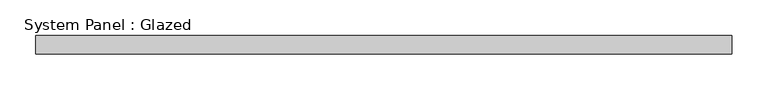
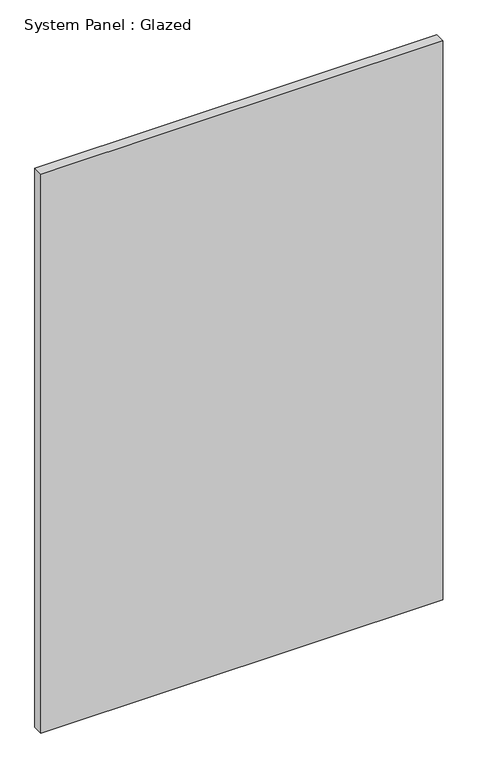
"""IFC4 building model written with IfcOpenShell, lengths in millimetres: plate geometry, System Panel : Glazed."""

from ifc_helpers import new_model, si_unit, origin, origin_with_axes, place, context, project, spatial, polyline, outline, extrude, source, transform, mapped, element, save


def system_panel_glazed_a8655be6(model_context):
    return source(origin(), model_context, "Body", "SweptSolid", [
        extrude(outline(polyline([(485.775, 19.05), (-485.775, 19.05), (-485.775, 44.45), (485.775, 44.45), (485.775, 19.05)])), origin_with_axes(), (0.0, 0.0, 1.0), 1428.75),
    ])


if __name__ == "__main__":
    model = new_model("IFC4")
    model_context = context("Model", 3, world=origin())
    ifc_project = project(units=[si_unit("LENGTHUNIT", "METRE", prefix="MILLI")], contexts=[model_context])
    site = spatial("IfcSite", under=ifc_project)
    building = spatial("IfcBuilding", under=site)
    placement = place(None, origin())
    system_panel_glazed_shape = system_panel_glazed_a8655be6(model_context)
    element("IfcPlate", 1, ObjectType="System Panel : Glazed", at=placement, inside=building, context=model_context, shape_type="MappedRepresentation", body=[
        mapped(system_panel_glazed_shape, transform((0.0, 0.0, 0.0), x_axis=(1.0, 0.0, 0.0), y_axis=(0.0, 1.0, 0.0), z_axis=(0.0, 0.0, 1.0))),
    ])
    save(model, "model.ifc")

# Revit data of these elements
# Type "System Panel : Glazed"
#   Construction Type Id = "GSP4R"
#   Analytic Construction = "1/8 in Pilkington single glazing"
#   Visual Light Transmittance = 0.9
#   Solar Heat Gain Coefficient = 0.86
#   Heat Transfer Coefficient (U) = 1.18115 BTU/(h·ft²·°F)
#   Define Thermal Properties by = 1
# Element 1 (IfcPlate, "System Panel : Glazed")
#   Materials on its faces: "Glass"
# Materials
#   "Glass": class "Glass", colour RGB 0 128 192, transparency 0.75, Description = "Soda Lime Glass", Cost = 0
